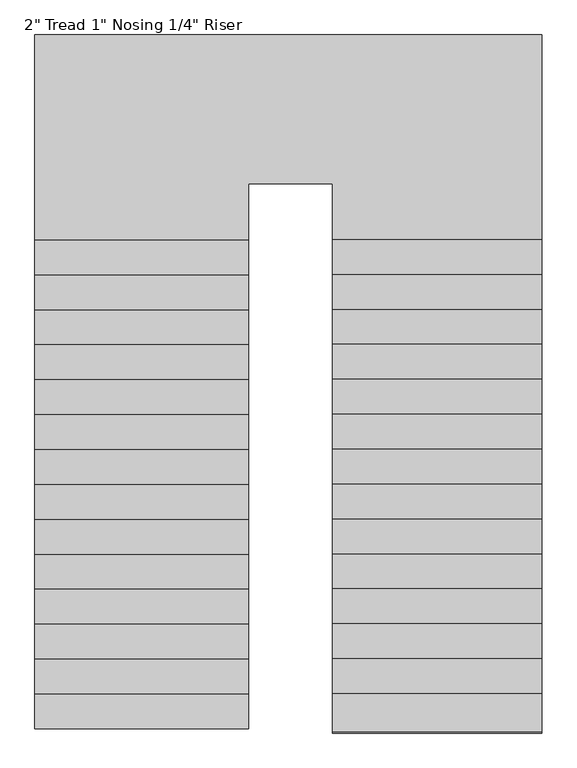
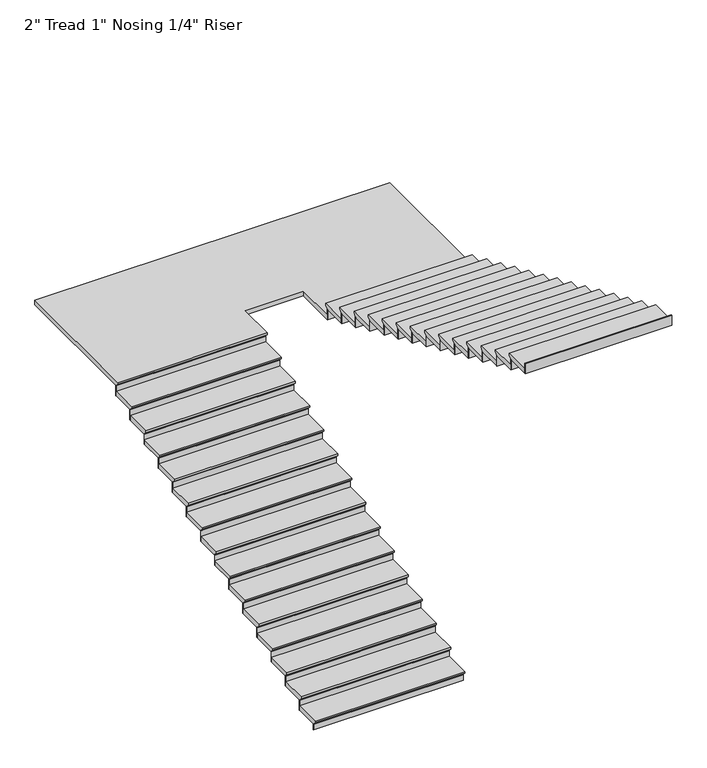
"""IFC4 building model written with IfcOpenShell, lengths in millimetres: stair flight geometry."""

from ifc_helpers import new_model, si_unit, origin, place, context, project, spatial, faceted_brep, source, transform, mapped, element, save


def stair_flight_371d2c9c(model_context):
    return source(origin(), model_context, "Body", "Brep", [
        faceted_brep([(-5999.9290366, -6973.0610642, 5883.91), (-5999.9290366, -6973.0610642, 5902.96), (-7554.4415084, -6973.0610642, 5902.96), (-7554.4415084, -6973.0610642, 5883.91), (-5999.9290366, -6947.6610642, 5858.51), (-7554.4415084, -6947.6610642, 5858.51), (-5999.9290366, -6693.6610642, 5902.96), (-7554.4415084, -6693.6610642, 5902.96), (-7554.4415084, -6947.6610642, 5852.16), (-7554.4415084, -6693.6610642, 5852.16), (-5999.9290366, -6693.6610642, 5852.16), (-5999.9290366, -6947.6610642, 5852.16)], [[[0, 1, 2, 3]], [[4, 0, 3, 5]], [[2, 1, 6, 7]], [[8, 9, 10, 11]], [[2, 7, 9, 8, 5, 3]], [[8, 11, 4, 5]], [[6, 1, 0, 4, 11, 10]], [[7, 6, 10, 9]]]),
        faceted_brep([(-5999.9290366, -6947.6610642, 5852.16), (-5999.9290366, -6947.6610642, 5791.2), (-5999.9290366, -6941.3110642, 5791.2), (-5999.9290366, -6941.3110642, 5852.16), (-7554.4415084, -6947.6610642, 5852.16), (-7554.4415084, -6941.3110642, 5852.16), (-7554.4415084, -6941.3110642, 5791.2), (-7554.4415084, -6947.6610642, 5791.2)], [[[0, 1, 2, 3]], [[4, 5, 6, 7]], [[1, 0, 4, 7]], [[2, 1, 7, 6]], [[3, 2, 6, 5]], [[0, 3, 5, 4]]]),
        faceted_brep([(-5999.9290366, -6693.6610642, 5963.92), (-5999.9290366, -6693.6610642, 5852.16), (-5999.9290366, -6687.3110642, 5852.16), (-5999.9290366, -6687.3110642, 5963.92), (-7554.4415084, -6693.6610642, 5963.92), (-7554.4415084, -6687.3110642, 5963.92), (-7554.4415084, -6687.3110642, 5852.16), (-7554.4415084, -6693.6610642, 5852.16)], [[[0, 1, 2, 3]], [[4, 5, 6, 7]], [[1, 0, 4, 7]], [[2, 1, 7, 6]], [[3, 2, 6, 5]], [[0, 3, 5, 4]]]),
        faceted_brep([(-7554.4415084, -6719.0610642, 6014.72), (-5999.9290366, -6719.0610642, 6014.72), (-5999.9290366, -6439.6610642, 6014.72), (-7554.4415084, -6439.6610642, 6014.72), (-7554.4415084, -6693.6610642, 5963.92), (-7554.4415084, -6439.6610642, 5963.92), (-5999.9290366, -6439.6610642, 5963.92), (-5999.9290366, -6693.6610642, 5963.92), (-7554.4415084, -6693.6610642, 5970.27), (-7554.4415084, -6719.0610642, 5995.67), (-5999.9290366, -6693.6610642, 5970.27), (-5999.9290366, -6719.0610642, 5995.67)], [[[0, 1, 2, 3]], [[4, 5, 6, 7]], [[0, 3, 5, 4, 8, 9]], [[4, 7, 10, 8]], [[2, 1, 11, 10, 7, 6]], [[3, 2, 6, 5]], [[11, 1, 0, 9]], [[10, 11, 9, 8]]]),
        faceted_brep([(-5999.9290366, -6439.6610642, 6075.68), (-5999.9290366, -6439.6610642, 5963.92), (-5999.9290366, -6433.3110642, 5963.92), (-5999.9290366, -6433.3110642, 6075.68), (-7554.4415084, -6439.6610642, 6075.68), (-7554.4415084, -6433.3110642, 6075.68), (-7554.4415084, -6433.3110642, 5963.92), (-7554.4415084, -6439.6610642, 5963.92)], [[[0, 1, 2, 3]], [[4, 5, 6, 7]], [[1, 0, 4, 7]], [[2, 1, 7, 6]], [[3, 2, 6, 5]], [[0, 3, 5, 4]]]),
        faceted_brep([(-7554.4415084, -6465.0610642, 6126.48), (-5999.9290366, -6465.0610642, 6126.48), (-5999.9290366, -6185.6610642, 6126.48), (-7554.4415084, -6185.6610642, 6126.48), (-7554.4415084, -6439.6610642, 6075.68), (-7554.4415084, -6185.6610642, 6075.68), (-5999.9290366, -6185.6610642, 6075.68), (-5999.9290366, -6439.6610642, 6075.68), (-7554.4415084, -6439.6610642, 6082.03), (-7554.4415084, -6465.0610642, 6107.43), (-5999.9290366, -6439.6610642, 6082.03), (-5999.9290366, -6465.0610642, 6107.43)], [[[0, 1, 2, 3]], [[4, 5, 6, 7]], [[0, 3, 5, 4, 8, 9]], [[4, 7, 10, 8]], [[2, 1, 11, 10, 7, 6]], [[3, 2, 6, 5]], [[11, 1, 0, 9]], [[10, 11, 9, 8]]]),
        faceted_brep([(-5999.9290366, -6185.6610642, 6187.44), (-5999.9290366, -6185.6610642, 6075.68), (-5999.9290366, -6179.3110642, 6075.68), (-5999.9290366, -6179.3110642, 6187.44), (-7554.4415084, -6185.6610642, 6187.44), (-7554.4415084, -6179.3110642, 6187.44), (-7554.4415084, -6179.3110642, 6075.68), (-7554.4415084, -6185.6610642, 6075.68)], [[[0, 1, 2, 3]], [[4, 5, 6, 7]], [[1, 0, 4, 7]], [[2, 1, 7, 6]], [[3, 2, 6, 5]], [[0, 3, 5, 4]]]),
        faceted_brep([(-7554.4415084, -6211.0610642, 6238.24), (-5999.9290366, -6211.0610642, 6238.24), (-5999.9290366, -5931.6610642, 6238.24), (-7554.4415084, -5931.6610642, 6238.24), (-7554.4415084, -6185.6610642, 6187.44), (-7554.4415084, -5931.6610642, 6187.44), (-5999.9290366, -5931.6610642, 6187.44), (-5999.9290366, -6185.6610642, 6187.44), (-7554.4415084, -6185.6610642, 6193.79), (-7554.4415084, -6211.0610642, 6219.19), (-5999.9290366, -6185.6610642, 6193.79), (-5999.9290366, -6211.0610642, 6219.19)], [[[0, 1, 2, 3]], [[4, 5, 6, 7]], [[0, 3, 5, 4, 8, 9]], [[4, 7, 10, 8]], [[2, 1, 11, 10, 7, 6]], [[3, 2, 6, 5]], [[11, 1, 0, 9]], [[10, 11, 9, 8]]]),
        faceted_brep([(-5999.9290366, -5931.6610642, 6299.2), (-5999.9290366, -5931.6610642, 6187.44), (-5999.9290366, -5925.3110642, 6187.44), (-5999.9290366, -5925.3110642, 6299.2), (-7554.4415084, -5931.6610642, 6299.2), (-7554.4415084, -5925.3110642, 6299.2), (-7554.4415084, -5925.3110642, 6187.44), (-7554.4415084, -5931.6610642, 6187.44)], [[[0, 1, 2, 3]], [[4, 5, 6, 7]], [[1, 0, 4, 7]], [[2, 1, 7, 6]], [[3, 2, 6, 5]], [[0, 3, 5, 4]]]),
        faceted_brep([(-7554.4415084, -5957.0610642, 6350.0), (-5999.9290366, -5957.0610642, 6350.0), (-5999.9290366, -5677.6610642, 6350.0), (-7554.4415084, -5677.6610642, 6350.0), (-7554.4415084, -5931.6610642, 6299.2), (-7554.4415084, -5677.6610642, 6299.2), (-5999.9290366, -5677.6610642, 6299.2), (-5999.9290366, -5931.6610642, 6299.2), (-7554.4415084, -5931.6610642, 6305.55), (-7554.4415084, -5957.0610642, 6330.95), (-5999.9290366, -5931.6610642, 6305.55), (-5999.9290366, -5957.0610642, 6330.95)], [[[0, 1, 2, 3]], [[4, 5, 6, 7]], [[0, 3, 5, 4, 8, 9]], [[4, 7, 10, 8]], [[2, 1, 11, 10, 7, 6]], [[3, 2, 6, 5]], [[11, 1, 0, 9]], [[10, 11, 9, 8]]]),
        faceted_brep([(-5999.9290366, -5677.6610642, 6410.96), (-5999.9290366, -5677.6610642, 6299.2), (-5999.9290366, -5671.3110642, 6299.2), (-5999.9290366, -5671.3110642, 6410.96), (-7554.4415084, -5677.6610642, 6410.96), (-7554.4415084, -5671.3110642, 6410.96), (-7554.4415084, -5671.3110642, 6299.2), (-7554.4415084, -5677.6610642, 6299.2)], [[[0, 1, 2, 3]], [[4, 5, 6, 7]], [[1, 0, 4, 7]], [[2, 1, 7, 6]], [[3, 2, 6, 5]], [[0, 3, 5, 4]]]),
        faceted_brep([(-7554.4415084, -5703.0610642, 6461.76), (-5999.9290366, -5703.0610642, 6461.76), (-5999.9290366, -5423.6610642, 6461.76), (-7554.4415084, -5423.6610642, 6461.76), (-7554.4415084, -5677.6610642, 6410.96), (-7554.4415084, -5423.6610642, 6410.96), (-5999.9290366, -5423.6610642, 6410.96), (-5999.9290366, -5677.6610642, 6410.96), (-7554.4415084, -5677.6610642, 6417.31), (-7554.4415084, -5703.0610642, 6442.71), (-5999.9290366, -5677.6610642, 6417.31), (-5999.9290366, -5703.0610642, 6442.71)], [[[0, 1, 2, 3]], [[4, 5, 6, 7]], [[0, 3, 5, 4, 8, 9]], [[4, 7, 10, 8]], [[2, 1, 11, 10, 7, 6]], [[3, 2, 6, 5]], [[11, 1, 0, 9]], [[10, 11, 9, 8]]]),
        faceted_brep([(-5999.9290366, -5423.6610642, 6522.72), (-5999.9290366, -5423.6610642, 6410.96), (-5999.9290366, -5417.3110642, 6410.96), (-5999.9290366, -5417.3110642, 6522.72), (-7554.4415084, -5423.6610642, 6522.72), (-7554.4415084, -5417.3110642, 6522.72), (-7554.4415084, -5417.3110642, 6410.96), (-7554.4415084, -5423.6610642, 6410.96)], [[[0, 1, 2, 3]], [[4, 5, 6, 7]], [[1, 0, 4, 7]], [[2, 1, 7, 6]], [[3, 2, 6, 5]], [[0, 3, 5, 4]]]),
        faceted_brep([(-7554.4415084, -5449.0610642, 6573.52), (-5999.9290366, -5449.0610642, 6573.52), (-5999.9290366, -5169.6610642, 6573.52), (-7554.4415084, -5169.6610642, 6573.52), (-7554.4415084, -5423.6610642, 6522.72), (-7554.4415084, -5169.6610642, 6522.72), (-5999.9290366, -5169.6610642, 6522.72), (-5999.9290366, -5423.6610642, 6522.72), (-7554.4415084, -5423.6610642, 6529.07), (-7554.4415084, -5449.0610642, 6554.47), (-5999.9290366, -5423.6610642, 6529.07), (-5999.9290366, -5449.0610642, 6554.47)], [[[0, 1, 2, 3]], [[4, 5, 6, 7]], [[0, 3, 5, 4, 8, 9]], [[4, 7, 10, 8]], [[2, 1, 11, 10, 7, 6]], [[3, 2, 6, 5]], [[11, 1, 0, 9]], [[10, 11, 9, 8]]]),
        faceted_brep([(-5999.9290366, -5169.6610642, 6634.48), (-5999.9290366, -5169.6610642, 6522.72), (-5999.9290366, -5163.3110642, 6522.72), (-5999.9290366, -5163.3110642, 6634.48), (-7554.4415084, -5169.6610642, 6634.48), (-7554.4415084, -5163.3110642, 6634.48), (-7554.4415084, -5163.3110642, 6522.72), (-7554.4415084, -5169.6610642, 6522.72)], [[[0, 1, 2, 3]], [[4, 5, 6, 7]], [[1, 0, 4, 7]], [[2, 1, 7, 6]], [[3, 2, 6, 5]], [[0, 3, 5, 4]]]),
        faceted_brep([(-7554.4415084, -5195.0610642, 6685.28), (-5999.9290366, -5195.0610642, 6685.28), (-5999.9290366, -4915.6610642, 6685.28), (-7554.4415084, -4915.6610642, 6685.28), (-7554.4415084, -5169.6610642, 6634.48), (-7554.4415084, -4915.6610642, 6634.48), (-5999.9290366, -4915.6610642, 6634.48), (-5999.9290366, -5169.6610642, 6634.48), (-7554.4415084, -5169.6610642, 6640.83), (-7554.4415084, -5195.0610642, 6666.23), (-5999.9290366, -5169.6610642, 6640.83), (-5999.9290366, -5195.0610642, 6666.23)], [[[0, 1, 2, 3]], [[4, 5, 6, 7]], [[0, 3, 5, 4, 8, 9]], [[4, 7, 10, 8]], [[2, 1, 11, 10, 7, 6]], [[3, 2, 6, 5]], [[11, 1, 0, 9]], [[10, 11, 9, 8]]]),
        faceted_brep([(-5999.9290366, -4915.6610642, 6746.24), (-5999.9290366, -4915.6610642, 6634.48), (-5999.9290366, -4909.3110642, 6634.48), (-5999.9290366, -4909.3110642, 6746.24), (-7554.4415084, -4915.6610642, 6746.24), (-7554.4415084, -4909.3110642, 6746.24), (-7554.4415084, -4909.3110642, 6634.48), (-7554.4415084, -4915.6610642, 6634.48)], [[[0, 1, 2, 3]], [[4, 5, 6, 7]], [[1, 0, 4, 7]], [[2, 1, 7, 6]], [[3, 2, 6, 5]], [[0, 3, 5, 4]]]),
        faceted_brep([(-7554.4415084, -4941.0610642, 6797.04), (-5999.9290366, -4941.0610642, 6797.04), (-5999.9290366, -4661.6610642, 6797.04), (-7554.4415084, -4661.6610642, 6797.04), (-7554.4415084, -4915.6610642, 6746.24), (-7554.4415084, -4661.6610642, 6746.24), (-5999.9290366, -4661.6610642, 6746.24), (-5999.9290366, -4915.6610642, 6746.24), (-7554.4415084, -4915.6610642, 6752.59), (-7554.4415084, -4941.0610642, 6777.99), (-5999.9290366, -4915.6610642, 6752.59), (-5999.9290366, -4941.0610642, 6777.99)], [[[0, 1, 2, 3]], [[4, 5, 6, 7]], [[0, 3, 5, 4, 8, 9]], [[4, 7, 10, 8]], [[2, 1, 11, 10, 7, 6]], [[3, 2, 6, 5]], [[11, 1, 0, 9]], [[10, 11, 9, 8]]]),
        faceted_brep([(-5999.9290366, -4661.6610642, 6858.0), (-5999.9290366, -4661.6610642, 6746.24), (-5999.9290366, -4655.3110642, 6746.24), (-5999.9290366, -4655.3110642, 6858.0), (-7554.4415084, -4661.6610642, 6858.0), (-7554.4415084, -4655.3110642, 6858.0), (-7554.4415084, -4655.3110642, 6746.24), (-7554.4415084, -4661.6610642, 6746.24)], [[[0, 1, 2, 3]], [[4, 5, 6, 7]], [[1, 0, 4, 7]], [[2, 1, 7, 6]], [[3, 2, 6, 5]], [[0, 3, 5, 4]]]),
        faceted_brep([(-7554.4415084, -4687.0610642, 6908.8), (-5999.9290366, -4687.0610642, 6908.8), (-5999.9290366, -4407.6610642, 6908.8), (-7554.4415084, -4407.6610642, 6908.8), (-7554.4415084, -4661.6610642, 6858.0), (-7554.4415084, -4407.6610642, 6858.0), (-5999.9290366, -4407.6610642, 6858.0), (-5999.9290366, -4661.6610642, 6858.0), (-7554.4415084, -4661.6610642, 6864.35), (-7554.4415084, -4687.0610642, 6889.75), (-5999.9290366, -4661.6610642, 6864.35), (-5999.9290366, -4687.0610642, 6889.75)], [[[0, 1, 2, 3]], [[4, 5, 6, 7]], [[0, 3, 5, 4, 8, 9]], [[4, 7, 10, 8]], [[2, 1, 11, 10, 7, 6]], [[3, 2, 6, 5]], [[11, 1, 0, 9]], [[10, 11, 9, 8]]]),
        faceted_brep([(-5999.9290366, -4407.6610642, 6969.76), (-5999.9290366, -4407.6610642, 6858.0), (-5999.9290366, -4401.3110642, 6858.0), (-5999.9290366, -4401.3110642, 6969.76), (-7554.4415084, -4407.6610642, 6969.76), (-7554.4415084, -4401.3110642, 6969.76), (-7554.4415084, -4401.3110642, 6858.0), (-7554.4415084, -4407.6610642, 6858.0)], [[[0, 1, 2, 3]], [[4, 5, 6, 7]], [[1, 0, 4, 7]], [[2, 1, 7, 6]], [[3, 2, 6, 5]], [[0, 3, 5, 4]]]),
        faceted_brep([(-7554.4415084, -4433.0610642, 7020.56), (-5999.9290366, -4433.0610642, 7020.56), (-5999.9290366, -4153.6610642, 7020.56), (-7554.4415084, -4153.6610642, 7020.56), (-7554.4415084, -4407.6610642, 6969.76), (-7554.4415084, -4153.6610642, 6969.76), (-5999.9290366, -4153.6610642, 6969.76), (-5999.9290366, -4407.6610642, 6969.76), (-7554.4415084, -4407.6610642, 6976.11), (-7554.4415084, -4433.0610642, 7001.51), (-5999.9290366, -4407.6610642, 6976.11), (-5999.9290366, -4433.0610642, 7001.51)], [[[0, 1, 2, 3]], [[4, 5, 6, 7]], [[0, 3, 5, 4, 8, 9]], [[4, 7, 10, 8]], [[2, 1, 11, 10, 7, 6]], [[3, 2, 6, 5]], [[11, 1, 0, 9]], [[10, 11, 9, 8]]]),
        faceted_brep([(-5999.9290366, -4153.6610642, 7081.52), (-5999.9290366, -4153.6610642, 6969.76), (-5999.9290366, -4147.3110642, 6969.76), (-5999.9290366, -4147.3110642, 7081.52), (-7554.4415084, -4153.6610642, 7081.52), (-7554.4415084, -4147.3110642, 7081.52), (-7554.4415084, -4147.3110642, 6969.76), (-7554.4415084, -4153.6610642, 6969.76)], [[[0, 1, 2, 3]], [[4, 5, 6, 7]], [[1, 0, 4, 7]], [[2, 1, 7, 6]], [[3, 2, 6, 5]], [[0, 3, 5, 4]]]),
        faceted_brep([(-7554.4415084, -4179.0610642, 7132.32), (-5999.9290366, -4179.0610642, 7132.32), (-5999.9290366, -3899.6610642, 7132.32), (-7554.4415084, -3899.6610642, 7132.32), (-7554.4415084, -4153.6610642, 7081.52), (-7554.4415084, -3899.6610642, 7081.52), (-5999.9290366, -3899.6610642, 7081.52), (-5999.9290366, -4153.6610642, 7081.52), (-7554.4415084, -4153.6610642, 7087.87), (-7554.4415084, -4179.0610642, 7113.27), (-5999.9290366, -4153.6610642, 7087.87), (-5999.9290366, -4179.0610642, 7113.27)], [[[0, 1, 2, 3]], [[4, 5, 6, 7]], [[0, 3, 5, 4, 8, 9]], [[4, 7, 10, 8]], [[2, 1, 11, 10, 7, 6]], [[3, 2, 6, 5]], [[11, 1, 0, 9]], [[10, 11, 9, 8]]]),
        faceted_brep([(-5999.9290366, -3899.6610642, 7193.28), (-5999.9290366, -3899.6610642, 7081.52), (-5999.9290366, -3893.3110642, 7081.52), (-5999.9290366, -3893.3110642, 7193.28), (-7554.4415084, -3899.6610642, 7193.28), (-7554.4415084, -3893.3110642, 7193.28), (-7554.4415084, -3893.3110642, 7081.52), (-7554.4415084, -3899.6610642, 7081.52)], [[[0, 1, 2, 3]], [[4, 5, 6, 7]], [[1, 0, 4, 7]], [[2, 1, 7, 6]], [[3, 2, 6, 5]], [[0, 3, 5, 4]]]),
        faceted_brep([(-7554.4415084, -3925.0610642, 7244.08), (-5999.9290366, -3925.0610642, 7244.08), (-5999.9290366, -3645.6610642, 7244.08), (-7554.4415084, -3645.6610642, 7244.08), (-7554.4415084, -3899.6610642, 7193.28), (-7554.4415084, -3645.6610642, 7193.28), (-5999.9290366, -3645.6610642, 7193.28), (-5999.9290366, -3899.6610642, 7193.28), (-7554.4415084, -3899.6610642, 7199.63), (-7554.4415084, -3925.0610642, 7225.03), (-5999.9290366, -3899.6610642, 7199.63), (-5999.9290366, -3925.0610642, 7225.03)], [[[0, 1, 2, 3]], [[4, 5, 6, 7]], [[0, 3, 5, 4, 8, 9]], [[4, 7, 10, 8]], [[2, 1, 11, 10, 7, 6]], [[3, 2, 6, 5]], [[11, 1, 0, 9]], [[10, 11, 9, 8]]]),
        faceted_brep([(-5999.9290366, -3645.6610642, 7305.04), (-5999.9290366, -3645.6610642, 7193.28), (-5999.9290366, -3639.3110642, 7193.28), (-5999.9290366, -3639.3110642, 7305.04), (-7554.4415084, -3645.6610642, 7305.04), (-7554.4415084, -3639.3110642, 7305.04), (-7554.4415084, -3639.3110642, 7193.28), (-7554.4415084, -3645.6610642, 7193.28)], [[[0, 1, 2, 3]], [[4, 5, 6, 7]], [[1, 0, 4, 7]], [[2, 1, 7, 6]], [[3, 2, 6, 5]], [[0, 3, 5, 4]]]),
        faceted_brep([(-7554.4415084, -3671.0610642, 7355.84), (-5999.9290366, -3671.0610642, 7355.84), (-5999.9290366, -3391.6610642, 7355.84), (-7554.4415084, -3391.6610642, 7355.84), (-7554.4415084, -3645.6610642, 7305.04), (-7554.4415084, -3391.6610642, 7305.04), (-5999.9290366, -3391.6610642, 7305.04), (-5999.9290366, -3645.6610642, 7305.04), (-7554.4415084, -3645.6610642, 7311.39), (-7554.4415084, -3671.0610642, 7336.79), (-5999.9290366, -3645.6610642, 7311.39), (-5999.9290366, -3671.0610642, 7336.79)], [[[0, 1, 2, 3]], [[4, 5, 6, 7]], [[0, 3, 5, 4, 8, 9]], [[4, 7, 10, 8]], [[2, 1, 11, 10, 7, 6]], [[3, 2, 6, 5]], [[11, 1, 0, 9]], [[10, 11, 9, 8]]]),
        faceted_brep([(-5999.9290366, -3391.6610642, 7416.8), (-5999.9290366, -3391.6610642, 7305.04), (-5999.9290366, -3385.3110642, 7305.04), (-5999.9290366, -3385.3110642, 7416.8), (-7554.4415084, -3391.6610642, 7416.8), (-7554.4415084, -3385.3110642, 7416.8), (-7554.4415084, -3385.3110642, 7305.04), (-7554.4415084, -3391.6610642, 7305.04)], [[[0, 1, 2, 3]], [[4, 5, 6, 7]], [[1, 0, 4, 7]], [[2, 1, 7, 6]], [[3, 2, 6, 5]], [[0, 3, 5, 4]]]),
        faceted_brep([(-3866.3290366, -3442.4610642, 7467.6), (-3866.3290366, -1928.4217109, 7467.6), (-7554.4415084, -1928.4217109, 7467.6), (-7554.4415084, -3417.0610642, 7467.6), (-5999.9290366, -3417.0610642, 7467.6), (-5999.9290366, -3010.6610642, 7467.6), (-5390.3290366, -3010.6610642, 7467.6), (-5390.3290366, -3442.4610642, 7467.6), (-3866.3290366, -1928.4217109, 7416.8), (-3866.3290366, -3442.4610642, 7416.8), (-5390.3290366, -3442.4610642, 7416.8), (-5390.3290366, -3010.6610642, 7416.8), (-5999.9290366, -3010.6610642, 7416.8), (-5999.9290366, -3391.6610642, 7416.8), (-7554.4415084, -3391.6610642, 7416.8), (-7554.4415084, -1928.4217109, 7416.8), (-7554.4415084, -3391.6610642, 7423.15), (-7554.4415084, -3417.0610642, 7448.55), (-5999.9290366, -3391.6610642, 7423.15), (-5999.9290366, -3417.0610642, 7448.55)], [[[0, 1, 2, 3, 4, 5, 6, 7]], [[8, 9, 10, 11, 12, 13, 14, 15]], [[1, 0, 9, 8]], [[2, 1, 8, 15]], [[3, 2, 15, 14, 16, 17]], [[14, 13, 18, 16]], [[5, 4, 19, 18, 13, 12]], [[6, 5, 12, 11]], [[7, 6, 11, 10]], [[0, 7, 10, 9]], [[19, 4, 3, 17]], [[18, 19, 17, 16]]]),
        faceted_brep([(-5390.3290366, -3442.4610642, 7528.56), (-5390.3290366, -3442.4610642, 7416.8), (-5390.3290366, -3448.8110642, 7416.8), (-5390.3290366, -3448.8110642, 7528.56), (-3866.3290366, -3442.4610642, 7528.56), (-3866.3290366, -3448.8110642, 7528.56), (-3866.3290366, -3448.8110642, 7416.8), (-3866.3290366, -3442.4610642, 7416.8)], [[[0, 1, 2, 3]], [[4, 5, 6, 7]], [[1, 0, 4, 7]], [[2, 1, 7, 6]], [[3, 2, 6, 5]], [[0, 3, 5, 4]]]),
        faceted_brep([(-3866.3290366, -3417.0610642, 7579.36), (-5390.3290366, -3417.0610642, 7579.36), (-5390.3290366, -3696.4610642, 7579.36), (-3866.3290366, -3696.4610642, 7579.36), (-3866.3290366, -3442.4610642, 7528.56), (-3866.3290366, -3696.4610642, 7528.56), (-5390.3290366, -3696.4610642, 7528.56), (-5390.3290366, -3442.4610642, 7528.56), (-3866.3290366, -3442.4610642, 7534.91), (-3866.3290366, -3417.0610642, 7560.31), (-5390.3290366, -3442.4610642, 7534.91), (-5390.3290366, -3417.0610642, 7560.31)], [[[0, 1, 2, 3]], [[4, 5, 6, 7]], [[0, 3, 5, 4, 8, 9]], [[4, 7, 10, 8]], [[2, 1, 11, 10, 7, 6]], [[3, 2, 6, 5]], [[11, 1, 0, 9]], [[10, 11, 9, 8]]]),
        faceted_brep([(-5390.3290366, -3696.4610642, 7640.32), (-5390.3290366, -3696.4610642, 7528.56), (-5390.3290366, -3702.8110642, 7528.56), (-5390.3290366, -3702.8110642, 7640.32), (-3866.3290366, -3696.4610642, 7640.32), (-3866.3290366, -3702.8110642, 7640.32), (-3866.3290366, -3702.8110642, 7528.56), (-3866.3290366, -3696.4610642, 7528.56)], [[[0, 1, 2, 3]], [[4, 5, 6, 7]], [[1, 0, 4, 7]], [[2, 1, 7, 6]], [[3, 2, 6, 5]], [[0, 3, 5, 4]]]),
        faceted_brep([(-3866.3290366, -3671.0610642, 7691.12), (-5390.3290366, -3671.0610642, 7691.12), (-5390.3290366, -3950.4610642, 7691.12), (-3866.3290366, -3950.4610642, 7691.12), (-3866.3290366, -3696.4610642, 7640.32), (-3866.3290366, -3950.4610642, 7640.32), (-5390.3290366, -3950.4610642, 7640.32), (-5390.3290366, -3696.4610642, 7640.32), (-3866.3290366, -3696.4610642, 7646.67), (-3866.3290366, -3671.0610642, 7672.07), (-5390.3290366, -3696.4610642, 7646.67), (-5390.3290366, -3671.0610642, 7672.07)], [[[0, 1, 2, 3]], [[4, 5, 6, 7]], [[0, 3, 5, 4, 8, 9]], [[4, 7, 10, 8]], [[2, 1, 11, 10, 7, 6]], [[3, 2, 6, 5]], [[11, 1, 0, 9]], [[10, 11, 9, 8]]]),
        faceted_brep([(-5390.3290366, -3950.4610642, 7752.08), (-5390.3290366, -3950.4610642, 7640.32), (-5390.3290366, -3956.8110642, 7640.32), (-5390.3290366, -3956.8110642, 7752.08), (-3866.3290366, -3950.4610642, 7752.08), (-3866.3290366, -3956.8110642, 7752.08), (-3866.3290366, -3956.8110642, 7640.32), (-3866.3290366, -3950.4610642, 7640.32)], [[[0, 1, 2, 3]], [[4, 5, 6, 7]], [[1, 0, 4, 7]], [[2, 1, 7, 6]], [[3, 2, 6, 5]], [[0, 3, 5, 4]]]),
        faceted_brep([(-3866.3290366, -3925.0610642, 7802.88), (-5390.3290366, -3925.0610642, 7802.88), (-5390.3290366, -4204.4610642, 7802.88), (-3866.3290366, -4204.4610642, 7802.88), (-3866.3290366, -3950.4610642, 7752.08), (-3866.3290366, -4204.4610642, 7752.08), (-5390.3290366, -4204.4610642, 7752.08), (-5390.3290366, -3950.4610642, 7752.08), (-3866.3290366, -3950.4610642, 7758.43), (-3866.3290366, -3925.0610642, 7783.83), (-5390.3290366, -3950.4610642, 7758.43), (-5390.3290366, -3925.0610642, 7783.83)], [[[0, 1, 2, 3]], [[4, 5, 6, 7]], [[0, 3, 5, 4, 8, 9]], [[4, 7, 10, 8]], [[2, 1, 11, 10, 7, 6]], [[3, 2, 6, 5]], [[11, 1, 0, 9]], [[10, 11, 9, 8]]]),
        faceted_brep([(-5390.3290366, -4204.4610642, 7863.84), (-5390.3290366, -4204.4610642, 7752.08), (-5390.3290366, -4210.8110642, 7752.08), (-5390.3290366, -4210.8110642, 7863.84), (-3866.3290366, -4204.4610642, 7863.84), (-3866.3290366, -4210.8110642, 7863.84), (-3866.3290366, -4210.8110642, 7752.08), (-3866.3290366, -4204.4610642, 7752.08)], [[[0, 1, 2, 3]], [[4, 5, 6, 7]], [[1, 0, 4, 7]], [[2, 1, 7, 6]], [[3, 2, 6, 5]], [[0, 3, 5, 4]]]),
        faceted_brep([(-3866.3290366, -4179.0610642, 7914.64), (-5390.3290366, -4179.0610642, 7914.64), (-5390.3290366, -4458.4610642, 7914.64), (-3866.3290366, -4458.4610642, 7914.64), (-3866.3290366, -4204.4610642, 7863.84), (-3866.3290366, -4458.4610642, 7863.84), (-5390.3290366, -4458.4610642, 7863.84), (-5390.3290366, -4204.4610642, 7863.84), (-3866.3290366, -4204.4610642, 7870.19), (-3866.3290366, -4179.0610642, 7895.59), (-5390.3290366, -4204.4610642, 7870.19), (-5390.3290366, -4179.0610642, 7895.59)], [[[0, 1, 2, 3]], [[4, 5, 6, 7]], [[0, 3, 5, 4, 8, 9]], [[4, 7, 10, 8]], [[2, 1, 11, 10, 7, 6]], [[3, 2, 6, 5]], [[11, 1, 0, 9]], [[10, 11, 9, 8]]]),
        faceted_brep([(-5390.3290366, -4458.4610642, 7975.6), (-5390.3290366, -4458.4610642, 7863.84), (-5390.3290366, -4464.8110642, 7863.84), (-5390.3290366, -4464.8110642, 7975.6), (-3866.3290366, -4458.4610642, 7975.6), (-3866.3290366, -4464.8110642, 7975.6), (-3866.3290366, -4464.8110642, 7863.84), (-3866.3290366, -4458.4610642, 7863.84)], [[[0, 1, 2, 3]], [[4, 5, 6, 7]], [[1, 0, 4, 7]], [[2, 1, 7, 6]], [[3, 2, 6, 5]], [[0, 3, 5, 4]]]),
        faceted_brep([(-3866.3290366, -4433.0610642, 8026.4), (-5390.3290366, -4433.0610642, 8026.4), (-5390.3290366, -4712.4610642, 8026.4), (-3866.3290366, -4712.4610642, 8026.4), (-3866.3290366, -4458.4610642, 7975.6), (-3866.3290366, -4712.4610642, 7975.6), (-5390.3290366, -4712.4610642, 7975.6), (-5390.3290366, -4458.4610642, 7975.6), (-3866.3290366, -4458.4610642, 7981.95), (-3866.3290366, -4433.0610642, 8007.35), (-5390.3290366, -4458.4610642, 7981.95), (-5390.3290366, -4433.0610642, 8007.35)], [[[0, 1, 2, 3]], [[4, 5, 6, 7]], [[0, 3, 5, 4, 8, 9]], [[4, 7, 10, 8]], [[2, 1, 11, 10, 7, 6]], [[3, 2, 6, 5]], [[11, 1, 0, 9]], [[10, 11, 9, 8]]]),
        faceted_brep([(-5390.3290366, -4712.4610642, 8087.36), (-5390.3290366, -4712.4610642, 7975.6), (-5390.3290366, -4718.8110642, 7975.6), (-5390.3290366, -4718.8110642, 8087.36), (-3866.3290366, -4712.4610642, 8087.36), (-3866.3290366, -4718.8110642, 8087.36), (-3866.3290366, -4718.8110642, 7975.6), (-3866.3290366, -4712.4610642, 7975.6)], [[[0, 1, 2, 3]], [[4, 5, 6, 7]], [[1, 0, 4, 7]], [[2, 1, 7, 6]], [[3, 2, 6, 5]], [[0, 3, 5, 4]]]),
        faceted_brep([(-3866.3290366, -4687.0610642, 8138.16), (-5390.3290366, -4687.0610642, 8138.16), (-5390.3290366, -4966.4610642, 8138.16), (-3866.3290366, -4966.4610642, 8138.16), (-3866.3290366, -4712.4610642, 8087.36), (-3866.3290366, -4966.4610642, 8087.36), (-5390.3290366, -4966.4610642, 8087.36), (-5390.3290366, -4712.4610642, 8087.36), (-3866.3290366, -4712.4610642, 8093.71), (-3866.3290366, -4687.0610642, 8119.11), (-5390.3290366, -4712.4610642, 8093.71), (-5390.3290366, -4687.0610642, 8119.11)], [[[0, 1, 2, 3]], [[4, 5, 6, 7]], [[0, 3, 5, 4, 8, 9]], [[4, 7, 10, 8]], [[2, 1, 11, 10, 7, 6]], [[3, 2, 6, 5]], [[11, 1, 0, 9]], [[10, 11, 9, 8]]]),
        faceted_brep([(-5390.3290366, -4966.4610642, 8199.12), (-5390.3290366, -4966.4610642, 8087.36), (-5390.3290366, -4972.8110642, 8087.36), (-5390.3290366, -4972.8110642, 8199.12), (-3866.3290366, -4966.4610642, 8199.12), (-3866.3290366, -4972.8110642, 8199.12), (-3866.3290366, -4972.8110642, 8087.36), (-3866.3290366, -4966.4610642, 8087.36)], [[[0, 1, 2, 3]], [[4, 5, 6, 7]], [[1, 0, 4, 7]], [[2, 1, 7, 6]], [[3, 2, 6, 5]], [[0, 3, 5, 4]]]),
        faceted_brep([(-3866.3290366, -4941.0610642, 8249.92), (-5390.3290366, -4941.0610642, 8249.92), (-5390.3290366, -5220.4610642, 8249.92), (-3866.3290366, -5220.4610642, 8249.92), (-3866.3290366, -4966.4610642, 8199.12), (-3866.3290366, -5220.4610642, 8199.12), (-5390.3290366, -5220.4610642, 8199.12), (-5390.3290366, -4966.4610642, 8199.12), (-3866.3290366, -4966.4610642, 8205.47), (-3866.3290366, -4941.0610642, 8230.87), (-5390.3290366, -4966.4610642, 8205.47), (-5390.3290366, -4941.0610642, 8230.87)], [[[0, 1, 2, 3]], [[4, 5, 6, 7]], [[0, 3, 5, 4, 8, 9]], [[4, 7, 10, 8]], [[2, 1, 11, 10, 7, 6]], [[3, 2, 6, 5]], [[11, 1, 0, 9]], [[10, 11, 9, 8]]]),
        faceted_brep([(-5390.3290366, -5220.4610642, 8310.88), (-5390.3290366, -5220.4610642, 8199.12), (-5390.3290366, -5226.8110642, 8199.12), (-5390.3290366, -5226.8110642, 8310.88), (-3866.3290366, -5220.4610642, 8310.88), (-3866.3290366, -5226.8110642, 8310.88), (-3866.3290366, -5226.8110642, 8199.12), (-3866.3290366, -5220.4610642, 8199.12)], [[[0, 1, 2, 3]], [[4, 5, 6, 7]], [[1, 0, 4, 7]], [[2, 1, 7, 6]], [[3, 2, 6, 5]], [[0, 3, 5, 4]]]),
        faceted_brep([(-3866.3290366, -5195.0610642, 8361.68), (-5390.3290366, -5195.0610642, 8361.68), (-5390.3290366, -5474.4610642, 8361.68), (-3866.3290366, -5474.4610642, 8361.68), (-3866.3290366, -5220.4610642, 8310.88), (-3866.3290366, -5474.4610642, 8310.88), (-5390.3290366, -5474.4610642, 8310.88), (-5390.3290366, -5220.4610642, 8310.88), (-3866.3290366, -5220.4610642, 8317.23), (-3866.3290366, -5195.0610642, 8342.63), (-5390.3290366, -5220.4610642, 8317.23), (-5390.3290366, -5195.0610642, 8342.63)], [[[0, 1, 2, 3]], [[4, 5, 6, 7]], [[0, 3, 5, 4, 8, 9]], [[4, 7, 10, 8]], [[2, 1, 11, 10, 7, 6]], [[3, 2, 6, 5]], [[11, 1, 0, 9]], [[10, 11, 9, 8]]]),
        faceted_brep([(-5390.3290366, -5474.4610642, 8422.64), (-5390.3290366, -5474.4610642, 8310.88), (-5390.3290366, -5480.8110642, 8310.88), (-5390.3290366, -5480.8110642, 8422.64), (-3866.3290366, -5474.4610642, 8422.64), (-3866.3290366, -5480.8110642, 8422.64), (-3866.3290366, -5480.8110642, 8310.88), (-3866.3290366, -5474.4610642, 8310.88)], [[[0, 1, 2, 3]], [[4, 5, 6, 7]], [[1, 0, 4, 7]], [[2, 1, 7, 6]], [[3, 2, 6, 5]], [[0, 3, 5, 4]]]),
        faceted_brep([(-3866.3290366, -5449.0610642, 8473.44), (-5390.3290366, -5449.0610642, 8473.44), (-5390.3290366, -5728.4610642, 8473.44), (-3866.3290366, -5728.4610642, 8473.44), (-3866.3290366, -5474.4610642, 8422.64), (-3866.3290366, -5728.4610642, 8422.64), (-5390.3290366, -5728.4610642, 8422.64), (-5390.3290366, -5474.4610642, 8422.64), (-3866.3290366, -5474.4610642, 8428.99), (-3866.3290366, -5449.0610642, 8454.39), (-5390.3290366, -5474.4610642, 8428.99), (-5390.3290366, -5449.0610642, 8454.39)], [[[0, 1, 2, 3]], [[4, 5, 6, 7]], [[0, 3, 5, 4, 8, 9]], [[4, 7, 10, 8]], [[2, 1, 11, 10, 7, 6]], [[3, 2, 6, 5]], [[11, 1, 0, 9]], [[10, 11, 9, 8]]]),
        faceted_brep([(-5390.3290366, -5728.4610642, 8534.4), (-5390.3290366, -5728.4610642, 8422.64), (-5390.3290366, -5734.8110642, 8422.64), (-5390.3290366, -5734.8110642, 8534.4), (-3866.3290366, -5728.4610642, 8534.4), (-3866.3290366, -5734.8110642, 8534.4), (-3866.3290366, -5734.8110642, 8422.64), (-3866.3290366, -5728.4610642, 8422.64)], [[[0, 1, 2, 3]], [[4, 5, 6, 7]], [[1, 0, 4, 7]], [[2, 1, 7, 6]], [[3, 2, 6, 5]], [[0, 3, 5, 4]]]),
        faceted_brep([(-3866.3290366, -5703.0610642, 8585.2), (-5390.3290366, -5703.0610642, 8585.2), (-5390.3290366, -5982.4610642, 8585.2), (-3866.3290366, -5982.4610642, 8585.2), (-3866.3290366, -5728.4610642, 8534.4), (-3866.3290366, -5982.4610642, 8534.4), (-5390.3290366, -5982.4610642, 8534.4), (-5390.3290366, -5728.4610642, 8534.4), (-3866.3290366, -5728.4610642, 8540.75), (-3866.3290366, -5703.0610642, 8566.15), (-5390.3290366, -5728.4610642, 8540.75), (-5390.3290366, -5703.0610642, 8566.15)], [[[0, 1, 2, 3]], [[4, 5, 6, 7]], [[0, 3, 5, 4, 8, 9]], [[4, 7, 10, 8]], [[2, 1, 11, 10, 7, 6]], [[3, 2, 6, 5]], [[11, 1, 0, 9]], [[10, 11, 9, 8]]]),
        faceted_brep([(-5390.3290366, -5982.4610642, 8646.16), (-5390.3290366, -5982.4610642, 8534.4), (-5390.3290366, -5988.8110642, 8534.4), (-5390.3290366, -5988.8110642, 8646.16), (-3866.3290366, -5982.4610642, 8646.16), (-3866.3290366, -5988.8110642, 8646.16), (-3866.3290366, -5988.8110642, 8534.4), (-3866.3290366, -5982.4610642, 8534.4)], [[[0, 1, 2, 3]], [[4, 5, 6, 7]], [[1, 0, 4, 7]], [[2, 1, 7, 6]], [[3, 2, 6, 5]], [[0, 3, 5, 4]]]),
        faceted_brep([(-3866.3290366, -5957.0610642, 8696.96), (-5390.3290366, -5957.0610642, 8696.96), (-5390.3290366, -6236.4610642, 8696.96), (-3866.3290366, -6236.4610642, 8696.96), (-3866.3290366, -5982.4610642, 8646.16), (-3866.3290366, -6236.4610642, 8646.16), (-5390.3290366, -6236.4610642, 8646.16), (-5390.3290366, -5982.4610642, 8646.16), (-3866.3290366, -5982.4610642, 8652.51), (-3866.3290366, -5957.0610642, 8677.91), (-5390.3290366, -5982.4610642, 8652.51), (-5390.3290366, -5957.0610642, 8677.91)], [[[0, 1, 2, 3]], [[4, 5, 6, 7]], [[0, 3, 5, 4, 8, 9]], [[4, 7, 10, 8]], [[2, 1, 11, 10, 7, 6]], [[3, 2, 6, 5]], [[11, 1, 0, 9]], [[10, 11, 9, 8]]]),
        faceted_brep([(-5390.3290366, -6236.4610642, 8757.92), (-5390.3290366, -6236.4610642, 8646.16), (-5390.3290366, -6242.8110642, 8646.16), (-5390.3290366, -6242.8110642, 8757.92), (-3866.3290366, -6236.4610642, 8757.92), (-3866.3290366, -6242.8110642, 8757.92), (-3866.3290366, -6242.8110642, 8646.16), (-3866.3290366, -6236.4610642, 8646.16)], [[[0, 1, 2, 3]], [[4, 5, 6, 7]], [[1, 0, 4, 7]], [[2, 1, 7, 6]], [[3, 2, 6, 5]], [[0, 3, 5, 4]]]),
        faceted_brep([(-3866.3290366, -6211.0610642, 8808.72), (-5390.3290366, -6211.0610642, 8808.72), (-5390.3290366, -6490.4610642, 8808.72), (-3866.3290366, -6490.4610642, 8808.72), (-3866.3290366, -6236.4610642, 8757.92), (-3866.3290366, -6490.4610642, 8757.92), (-5390.3290366, -6490.4610642, 8757.92), (-5390.3290366, -6236.4610642, 8757.92), (-3866.3290366, -6236.4610642, 8764.27), (-3866.3290366, -6211.0610642, 8789.67), (-5390.3290366, -6236.4610642, 8764.27), (-5390.3290366, -6211.0610642, 8789.67)], [[[0, 1, 2, 3]], [[4, 5, 6, 7]], [[0, 3, 5, 4, 8, 9]], [[4, 7, 10, 8]], [[2, 1, 11, 10, 7, 6]], [[3, 2, 6, 5]], [[11, 1, 0, 9]], [[10, 11, 9, 8]]]),
        faceted_brep([(-5390.3290366, -6490.4610642, 8869.68), (-5390.3290366, -6490.4610642, 8757.92), (-5390.3290366, -6496.8110642, 8757.92), (-5390.3290366, -6496.8110642, 8869.68), (-3866.3290366, -6490.4610642, 8869.68), (-3866.3290366, -6496.8110642, 8869.68), (-3866.3290366, -6496.8110642, 8757.92), (-3866.3290366, -6490.4610642, 8757.92)], [[[0, 1, 2, 3]], [[4, 5, 6, 7]], [[1, 0, 4, 7]], [[2, 1, 7, 6]], [[3, 2, 6, 5]], [[0, 3, 5, 4]]]),
        faceted_brep([(-3866.3290366, -6465.0610642, 8920.48), (-5390.3290366, -6465.0610642, 8920.48), (-5390.3290366, -6744.4610642, 8920.48), (-3866.3290366, -6744.4610642, 8920.48), (-3866.3290366, -6490.4610642, 8869.68), (-3866.3290366, -6744.4610642, 8869.68), (-5390.3290366, -6744.4610642, 8869.68), (-5390.3290366, -6490.4610642, 8869.68), (-3866.3290366, -6490.4610642, 8876.03), (-3866.3290366, -6465.0610642, 8901.43), (-5390.3290366, -6490.4610642, 8876.03), (-5390.3290366, -6465.0610642, 8901.43)], [[[0, 1, 2, 3]], [[4, 5, 6, 7]], [[0, 3, 5, 4, 8, 9]], [[4, 7, 10, 8]], [[2, 1, 11, 10, 7, 6]], [[3, 2, 6, 5]], [[11, 1, 0, 9]], [[10, 11, 9, 8]]]),
        faceted_brep([(-5390.3290366, -6744.4610642, 8981.44), (-5390.3290366, -6744.4610642, 8869.68), (-5390.3290366, -6750.8110642, 8869.68), (-5390.3290366, -6750.8110642, 8981.44), (-3866.3290366, -6744.4610642, 8981.44), (-3866.3290366, -6750.8110642, 8981.44), (-3866.3290366, -6750.8110642, 8869.68), (-3866.3290366, -6744.4610642, 8869.68)], [[[0, 1, 2, 3]], [[4, 5, 6, 7]], [[1, 0, 4, 7]], [[2, 1, 7, 6]], [[3, 2, 6, 5]], [[0, 3, 5, 4]]]),
        faceted_brep([(-5390.3290366, -6998.4610642, 9093.2), (-5390.3290366, -6998.4610642, 8981.44), (-5390.3290366, -7004.8110642, 8981.44), (-5390.3290366, -7004.8110642, 9093.2), (-3866.3290366, -6998.4610642, 9093.2), (-3866.3290366, -7004.8110642, 9093.2), (-3866.3290366, -7004.8110642, 8981.44), (-3866.3290366, -6998.4610642, 8981.44)], [[[0, 1, 2, 3]], [[4, 5, 6, 7]], [[1, 0, 4, 7]], [[2, 1, 7, 6]], [[3, 2, 6, 5]], [[0, 3, 5, 4]]]),
        faceted_brep([(-3866.3290366, -6719.0610642, 9032.24), (-5390.3290366, -6719.0610642, 9032.24), (-5390.3290366, -6998.4610642, 9032.24), (-3866.3290366, -6998.4610642, 9032.24), (-3866.3290366, -6744.4610642, 8981.44), (-3866.3290366, -6998.4610642, 8981.44), (-5390.3290366, -6998.4610642, 8981.44), (-5390.3290366, -6744.4610642, 8981.44), (-3866.3290366, -6744.4610642, 8987.79), (-3866.3290366, -6719.0610642, 9013.19), (-5390.3290366, -6744.4610642, 8987.79), (-5390.3290366, -6719.0610642, 9013.19)], [[[0, 1, 2, 3]], [[4, 5, 6, 7]], [[0, 3, 5, 4, 8, 9]], [[4, 7, 10, 8]], [[2, 1, 11, 10, 7, 6]], [[3, 2, 6, 5]], [[11, 1, 0, 9]], [[10, 11, 9, 8]]]),
    ])


if __name__ == "__main__":
    model = new_model("IFC4")
    model_context = context("Model", 3, world=origin())
    ifc_project = project(units=[si_unit("LENGTHUNIT", "METRE", prefix="MILLI")], contexts=[model_context])
    site = spatial("IfcSite", under=ifc_project)
    building = spatial("IfcBuilding", under=site)
    placement = place(None, origin())
    stair_flight_shape = stair_flight_371d2c9c(model_context)
    element("IfcStairFlight", 1, ObjectType="2\" Tread 1\" Nosing 1/4\" Riser", at=placement, inside=building, context=model_context, shape_type="MappedRepresentation", body=[
        mapped(stair_flight_shape, transform((0.0, 0.0, 0.0), x_axis=(1.0, 0.0, 0.0), y_axis=(0.0, 1.0, 0.0), z_axis=(0.0, 0.0, 1.0))),
    ])
    save(model, "model.ifc")
